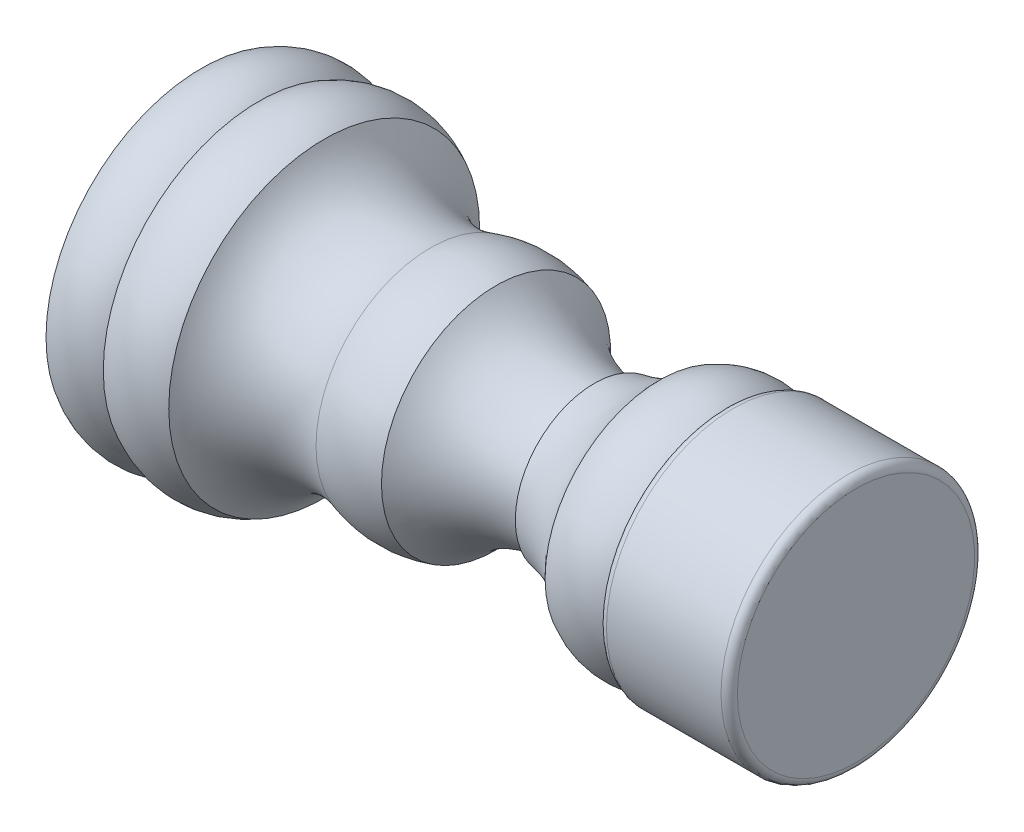
ISO-10303-21;
HEADER;
FILE_DESCRIPTION(('STEP AP214'),'2;1');
FILE_NAME('part.step','',(''),(''),'','','');
FILE_SCHEMA(('AUTOMOTIVE_DESIGN { 1 0 10303 214 1 1 1 1 }'));
ENDSEC;
DATA;
#1=APPLICATION_CONTEXT('core data for automotive mechanical design processes');
#2=APPLICATION_PROTOCOL_DEFINITION('international standard','automotive_design',2000,#1);
#3=PRODUCT_CONTEXT('',#1,'mechanical');
#4=PRODUCT('Part','Part','',(#3));
#5=PRODUCT_RELATED_PRODUCT_CATEGORY('part','',(#4));
#6=PRODUCT_DEFINITION_FORMATION('','',#4);
#7=PRODUCT_DEFINITION_CONTEXT('part definition',#1,'design');
#8=PRODUCT_DEFINITION('design','',#6,#7);
#9=PRODUCT_DEFINITION_SHAPE('','',#8);
#10=(LENGTH_UNIT() NAMED_UNIT(*) SI_UNIT(.MILLI.,.METRE.));
#11=(NAMED_UNIT(*) PLANE_ANGLE_UNIT() SI_UNIT($,.RADIAN.));
#12=(NAMED_UNIT(*) SI_UNIT($,.STERADIAN.) SOLID_ANGLE_UNIT());
#13=UNCERTAINTY_MEASURE_WITH_UNIT(LENGTH_MEASURE(1.E-05),#10,'distance_accuracy_value','');
#14=(GEOMETRIC_REPRESENTATION_CONTEXT(3) GLOBAL_UNCERTAINTY_ASSIGNED_CONTEXT((#13)) GLOBAL_UNIT_ASSIGNED_CONTEXT((#10,
#11,#12)) REPRESENTATION_CONTEXT('',''));
#15=CARTESIAN_POINT('',(0.,0.,0.));
#16=DIRECTION('',(0.,0.,1.));
#17=DIRECTION('',(1.,0.,0.));
#18=AXIS2_PLACEMENT_3D('',#15,#16,#17);
#19=CARTESIAN_POINT('',(0.,0.,0.));
#20=DIRECTION('',(-1.,0.,0.));
#21=DIRECTION('',(0.,0.,1.));
#22=AXIS2_PLACEMENT_3D('',#19,#20,#21);
#23=PLANE('',#22);
#24=CARTESIAN_POINT('',(0.,0.,0.));
#25=DIRECTION('',(-1.,0.,0.));
#26=DIRECTION('',(0.,0.,1.));
#27=AXIS2_PLACEMENT_3D('',#24,#25,#26);
#28=CIRCLE('',#27,14.25);
#29=CARTESIAN_POINT('',(0.,0.,14.25));
#30=VERTEX_POINT('',#29);
#31=EDGE_CURVE('E78',#30,#30,#28,.T.);
#32=ORIENTED_EDGE('',*,*,#31,.T.);
#33=EDGE_LOOP('',(#32));
#34=FACE_BOUND('',#33,.T.);
#35=ADVANCED_FACE('F40',(#34),#23,.T.);
#36=CARTESIAN_POINT('',(60.,0.,0.));
#37=DIRECTION('',(-1.,0.,0.));
#38=DIRECTION('',(0.,0.,1.));
#39=AXIS2_PLACEMENT_3D('',#36,#37,#38);
#40=PLANE('',#39);
#41=CARTESIAN_POINT('',(60.,0.,0.));
#42=DIRECTION('',(-1.,0.,0.));
#43=DIRECTION('',(0.,0.,1.));
#44=AXIS2_PLACEMENT_3D('',#41,#42,#43);
#45=CIRCLE('',#44,10.875);
#46=CARTESIAN_POINT('',(60.,0.,10.875));
#47=VERTEX_POINT('',#46);
#48=EDGE_CURVE('E10',#47,#47,#45,.T.);
#49=ORIENTED_EDGE('',*,*,#48,.F.);
#50=EDGE_LOOP('',(#49));
#51=FACE_BOUND('',#50,.T.);
#52=ADVANCED_FACE('F108',(#51),#40,.F.);
#53=CARTESIAN_POINT('',(59.25,0.,0.));
#54=DIRECTION('',(-1.,0.,0.));
#55=DIRECTION('',(0.,0.,1.));
#56=AXIS2_PLACEMENT_3D('',#53,#54,#55);
#57=TOROIDAL_SURFACE('',#56,10.875,0.750000000000001);
#58=CARTESIAN_POINT('',(59.25,0.,0.));
#59=DIRECTION('',(-1.,0.,0.));
#60=DIRECTION('',(0.,0.,1.));
#61=AXIS2_PLACEMENT_3D('',#58,#59,#60);
#62=CIRCLE('',#61,11.625);
#63=CARTESIAN_POINT('',(59.25,0.,11.625));
#64=VERTEX_POINT('',#63);
#65=EDGE_CURVE('E43',#64,#64,#62,.T.);
#66=ORIENTED_EDGE('',*,*,#65,.F.);
#67=EDGE_LOOP('',(#66));
#68=FACE_BOUND('',#67,.T.);
#69=ORIENTED_EDGE('',*,*,#48,.T.);
#70=EDGE_LOOP('',(#69));
#71=FACE_BOUND('',#70,.T.);
#72=ADVANCED_FACE('F114',(#68,#71),#57,.T.);
#73=CARTESIAN_POINT('',(0.,0.,0.));
#74=DIRECTION('',(-1.,0.,0.));
#75=DIRECTION('',(0.,0.,1.));
#76=AXIS2_PLACEMENT_3D('',#73,#74,#75);
#77=CYLINDRICAL_SURFACE('',#76,11.625);
#78=CARTESIAN_POINT('',(48.75,0.,0.));
#79=DIRECTION('',(-1.,0.,0.));
#80=DIRECTION('',(0.,0.,1.));
#81=AXIS2_PLACEMENT_3D('',#78,#79,#80);
#82=CIRCLE('',#81,11.625);
#83=CARTESIAN_POINT('',(48.75,0.,11.625));
#84=VERTEX_POINT('',#83);
#85=EDGE_CURVE('E50',#84,#84,#82,.T.);
#86=ORIENTED_EDGE('',*,*,#85,.F.);
#87=EDGE_LOOP('',(#86));
#88=FACE_BOUND('',#87,.T.);
#89=ORIENTED_EDGE('',*,*,#65,.T.);
#90=EDGE_LOOP('',(#89));
#91=FACE_BOUND('',#90,.T.);
#92=ADVANCED_FACE('F119',(#88,#91),#77,.T.);
#93=CARTESIAN_POINT('',(48.75,0.,0.));
#94=DIRECTION('',(-1.,0.,0.));
#95=DIRECTION('',(0.,0.,1.));
#96=AXIS2_PLACEMENT_3D('',#93,#94,#95);
#97=TOROIDAL_SURFACE('',#96,10.875,0.750000000000001);
#98=CARTESIAN_POINT('',(48.,0.,0.));
#99=DIRECTION('',(-1.,0.,0.));
#100=DIRECTION('',(0.,0.,1.));
#101=AXIS2_PLACEMENT_3D('',#98,#99,#100);
#102=CIRCLE('',#101,10.875);
#103=CARTESIAN_POINT('',(48.,0.,10.875));
#104=VERTEX_POINT('',#103);
#105=EDGE_CURVE('E51',#104,#104,#102,.T.);
#106=ORIENTED_EDGE('',*,*,#105,.F.);
#107=EDGE_LOOP('',(#106));
#108=FACE_BOUND('',#107,.T.);
#109=ORIENTED_EDGE('',*,*,#85,.T.);
#110=EDGE_LOOP('',(#109));
#111=FACE_BOUND('',#110,.T.);
#112=ADVANCED_FACE('F123',(#108,#111),#97,.T.);
#113=CARTESIAN_POINT('',(48.,10.5,0.));
#114=DIRECTION('',(-1.,0.,0.));
#115=DIRECTION('',(0.,0.,1.));
#116=AXIS2_PLACEMENT_3D('',#113,#114,#115);
#117=PLANE('',#116);
#118=ORIENTED_EDGE('',*,*,#105,.T.);
#119=EDGE_LOOP('',(#118));
#120=FACE_BOUND('',#119,.T.);
#121=CARTESIAN_POINT('',(48.,0.,0.));
#122=DIRECTION('',(-1.,0.,0.));
#123=DIRECTION('',(0.,0.,1.));
#124=AXIS2_PLACEMENT_3D('',#121,#122,#123);
#125=CIRCLE('',#124,10.5);
#126=CARTESIAN_POINT('',(48.,0.,10.5));
#127=VERTEX_POINT('',#126);
#128=EDGE_CURVE('E57',#127,#127,#125,.T.);
#129=ORIENTED_EDGE('',*,*,#128,.F.);
#130=EDGE_LOOP('',(#129));
#131=FACE_BOUND('',#130,.T.);
#132=ADVANCED_FACE('F126',(#120,#131),#117,.T.);
#133=CARTESIAN_POINT('',(45.,0.,0.));
#134=DIRECTION('',(-1.,0.,0.));
#135=DIRECTION('',(0.,0.,1.));
#136=AXIS2_PLACEMENT_3D('',#133,#134,#135);
#137=DEGENERATE_TOROIDAL_SURFACE('',#136,5.2174225041179,6.075,.T.);
#138=CARTESIAN_POINT('',(42.,0.,0.));
#139=DIRECTION('',(-1.,0.,0.));
#140=DIRECTION('',(0.,0.,1.));
#141=AXIS2_PLACEMENT_3D('',#138,#139,#140);
#142=CIRCLE('',#141,10.5);
#143=CARTESIAN_POINT('',(42.,0.,10.5));
#144=VERTEX_POINT('',#143);
#145=EDGE_CURVE('E56',#144,#144,#142,.T.);
#146=ORIENTED_EDGE('',*,*,#145,.F.);
#147=EDGE_LOOP('',(#146));
#148=FACE_BOUND('',#147,.T.);
#149=ORIENTED_EDGE('',*,*,#128,.T.);
#150=EDGE_LOOP('',(#149));
#151=FACE_BOUND('',#150,.T.);
#152=ADVANCED_FACE('F135',(#148,#151),#137,.T.);
#153=CARTESIAN_POINT('',(34.6453719233449,0.,0.));
#154=DIRECTION('',(-1.,0.,0.));
#155=DIRECTION('',(0.,0.,1.));
#156=AXIS2_PLACEMENT_3D('',#153,#154,#155);
#157=TOROIDAL_SURFACE('',#156,16.8551432599176,9.72);
#158=ORIENTED_EDGE('',*,*,#145,.T.);
#159=EDGE_LOOP('',(#158));
#160=FACE_BOUND('',#159,.T.);
#161=CARTESIAN_POINT('',(36.,0.,0.));
#162=DIRECTION('',(-1.,0.,0.));
#163=DIRECTION('',(0.,0.,1.));
#164=AXIS2_PLACEMENT_3D('',#161,#162,#163);
#165=CIRCLE('',#164,7.23);
#166=CARTESIAN_POINT('',(36.,0.,7.23));
#167=VERTEX_POINT('',#166);
#168=EDGE_CURVE('E65',#167,#167,#165,.T.);
#169=ORIENTED_EDGE('',*,*,#168,.F.);
#170=EDGE_LOOP('',(#169));
#171=FACE_BOUND('',#170,.T.);
#172=ADVANCED_FACE('F139',(#160,#171),#157,.F.);
#173=CARTESIAN_POINT('',(36.,7.23,0.));
#174=DIRECTION('',(1.,0.,0.));
#175=DIRECTION('',(0.,0.,-1.));
#176=AXIS2_PLACEMENT_3D('',#173,#174,#175);
#177=PLANE('',#176);
#178=CARTESIAN_POINT('',(36.,0.,0.));
#179=DIRECTION('',(-1.,0.,0.));
#180=DIRECTION('',(0.,0.,1.));
#181=AXIS2_PLACEMENT_3D('',#178,#179,#180);
#182=CIRCLE('',#181,6.48);
#183=CARTESIAN_POINT('',(36.,0.,6.48));
#184=VERTEX_POINT('',#183);
#185=EDGE_CURVE('E63',#184,#184,#182,.T.);
#186=ORIENTED_EDGE('',*,*,#185,.F.);
#187=EDGE_LOOP('',(#186));
#188=FACE_BOUND('',#187,.T.);
#189=ORIENTED_EDGE('',*,*,#168,.T.);
#190=EDGE_LOOP('',(#189));
#191=FACE_BOUND('',#190,.T.);
#192=ADVANCED_FACE('F137',(#188,#191),#177,.F.);
#193=CARTESIAN_POINT('',(35.6651918570158,0.,0.));
#194=DIRECTION('',(-1.,0.,0.));
#195=DIRECTION('',(0.,0.,1.));
#196=AXIS2_PLACEMENT_3D('',#193,#194,#195);
#197=TOROIDAL_SURFACE('',#196,17.815056396304,11.34);
#198=ORIENTED_EDGE('',*,*,#185,.T.);
#199=EDGE_LOOP('',(#198));
#200=FACE_BOUND('',#199,.T.);
#201=CARTESIAN_POINT('',(27.,0.,0.));
#202=DIRECTION('',(-1.,0.,0.));
#203=DIRECTION('',(0.,0.,1.));
#204=AXIS2_PLACEMENT_3D('',#201,#202,#203);
#205=CIRCLE('',#204,10.5);
#206=CARTESIAN_POINT('',(27.,0.,10.5));
#207=VERTEX_POINT('',#206);
#208=EDGE_CURVE('E70',#207,#207,#205,.T.);
#209=ORIENTED_EDGE('',*,*,#208,.F.);
#210=EDGE_LOOP('',(#209));
#211=FACE_BOUND('',#210,.T.);
#212=ADVANCED_FACE('F104',(#200,#211),#197,.F.);
#213=CARTESIAN_POINT('',(24.,0.,0.));
#214=DIRECTION('',(-1.,0.,0.));
#215=DIRECTION('',(0.,0.,1.));
#216=AXIS2_PLACEMENT_3D('',#213,#214,#215);
#217=DEGENERATE_TOROIDAL_SURFACE('',#216,0.892491217802611,10.065,.T.);
#218=CARTESIAN_POINT('',(21.,0.,0.));
#219=DIRECTION('',(-1.,0.,0.));
#220=DIRECTION('',(0.,0.,1.));
#221=AXIS2_PLACEMENT_3D('',#218,#219,#220);
#222=CIRCLE('',#221,10.5);
#223=CARTESIAN_POINT('',(21.,0.,10.5));
#224=VERTEX_POINT('',#223);
#225=EDGE_CURVE('E72',#224,#224,#222,.T.);
#226=ORIENTED_EDGE('',*,*,#225,.F.);
#227=EDGE_LOOP('',(#226));
#228=FACE_BOUND('',#227,.T.);
#229=ORIENTED_EDGE('',*,*,#208,.T.);
#230=EDGE_LOOP('',(#229));
#231=FACE_BOUND('',#230,.T.);
#232=ADVANCED_FACE('F97',(#228,#231),#217,.T.);
#233=CARTESIAN_POINT('',(18.2907821020135,0.,0.));
#234=DIRECTION('',(-1.,0.,0.));
#235=DIRECTION('',(0.,0.,1.));
#236=AXIS2_PLACEMENT_3D('',#233,#234,#235);
#237=TOROIDAL_SURFACE('',#236,18.0060334652351,7.98);
#238=ORIENTED_EDGE('',*,*,#225,.T.);
#239=EDGE_LOOP('',(#238));
#240=FACE_BOUND('',#239,.T.);
#241=CARTESIAN_POINT('',(11.25,0.,0.));
#242=DIRECTION('',(-1.,0.,0.));
#243=DIRECTION('',(0.,0.,1.));
#244=AXIS2_PLACEMENT_3D('',#241,#242,#243);
#245=CIRCLE('',#244,14.25);
#246=CARTESIAN_POINT('',(11.25,0.,14.25));
#247=VERTEX_POINT('',#246);
#248=EDGE_CURVE('E74',#247,#247,#245,.T.);
#249=ORIENTED_EDGE('',*,*,#248,.F.);
#250=EDGE_LOOP('',(#249));
#251=FACE_BOUND('',#250,.T.);
#252=ADVANCED_FACE('F94',(#240,#251),#237,.F.);
#253=CARTESIAN_POINT('',(8.25000000000002,0.,0.));
#254=DIRECTION('',(-1.,0.,0.));
#255=DIRECTION('',(0.,0.,1.));
#256=AXIS2_PLACEMENT_3D('',#253,#254,#255);
#257=TOROIDAL_SURFACE('',#256,8.88134094954802,6.15);
#258=CARTESIAN_POINT('',(5.25000000000002,0.,0.));
#259=DIRECTION('',(-1.,0.,0.));
#260=DIRECTION('',(0.,0.,1.));
#261=AXIS2_PLACEMENT_3D('',#258,#259,#260);
#262=CIRCLE('',#261,14.25);
#263=CARTESIAN_POINT('',(5.25000000000002,0.,14.25));
#264=VERTEX_POINT('',#263);
#265=EDGE_CURVE('E80',#264,#264,#262,.T.);
#266=ORIENTED_EDGE('',*,*,#265,.F.);
#267=EDGE_LOOP('',(#266));
#268=FACE_BOUND('',#267,.T.);
#269=ORIENTED_EDGE('',*,*,#248,.T.);
#270=EDGE_LOOP('',(#269));
#271=FACE_BOUND('',#270,.T.);
#272=ADVANCED_FACE('F86',(#268,#271),#257,.T.);
#273=CARTESIAN_POINT('',(2.625,0.,0.));
#274=DIRECTION('',(-1.,0.,0.));
#275=DIRECTION('',(0.,0.,1.));
#276=AXIS2_PLACEMENT_3D('',#273,#274,#275);
#277=TOROIDAL_SURFACE('',#276,10.0533495499387,4.95);
#278=ORIENTED_EDGE('',*,*,#31,.F.);
#279=EDGE_LOOP('',(#278));
#280=FACE_BOUND('',#279,.T.);
#281=ORIENTED_EDGE('',*,*,#265,.T.);
#282=EDGE_LOOP('',(#281));
#283=FACE_BOUND('',#282,.T.);
#284=ADVANCED_FACE('F82',(#280,#283),#277,.T.);
#285=CLOSED_SHELL('',(#35,#52,#72,#92,#112,#132,#152,#172,#192,#212,#232,#252,#272,#284));
#286=MANIFOLD_SOLID_BREP('B2',#285);
#287=ADVANCED_BREP_SHAPE_REPRESENTATION('',(#18,#286),#14);
#288=SHAPE_DEFINITION_REPRESENTATION(#9,#287);
ENDSEC;
END-ISO-10303-21;
